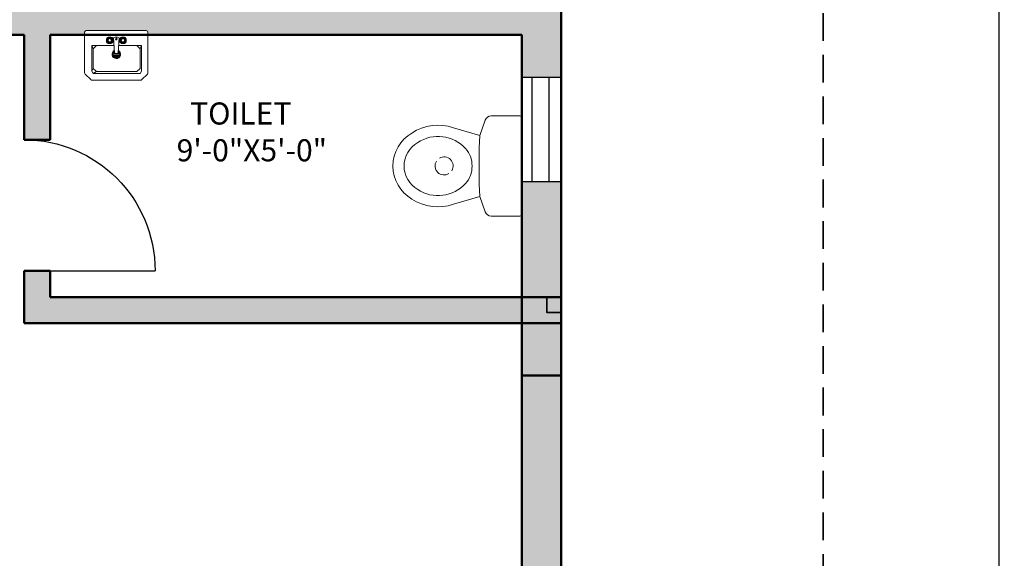
# Model space of a CAD drawing. Units: inches. Extents: x -7 to 1228, y -146 to 1091.
# Tile 86 of 88: x 1003 to 1228, y 691 to 814. Entities that reach past the tile are written whole.
import ezdxf

# ---------------------------------------------------------------- set-up
doc = ezdxf.new("R2010")
doc.units = ezdxf.units.IN
doc.linetypes.add('DASHED2', pattern=[9.525, 6.35, -3.175])
for name, color, linetype, lineweight in [('A-ANNO-DIMS', 2, 'Continuous', 18), ('A-AREA-IDEN', 7, 'Continuous', 18), ('A-COLS', 6, 'Continuous', 35), ('A-DOOR', 4, 'Continuous', 25), ('A-FLOR-FIXT', 8, 'Continuous', 18), ('A-FURN', 8, 'Continuous', 18), ('A-GLAZ', 175, 'Continuous', 25), ('A-WALL', 7, 'Continuous', 50), ('A-WALL-PATT', 251, 'Continuous', 13), ('C-PROP', 1, 'DASHED2', 35)]:
    doc.layers.add(name, color=color, linetype=linetype, lineweight=lineweight)
doc.styles.get("Standard").update_dxf_attribs({"font": 'arial.ttf'})
doc.dimstyles.new('ISO-25', dxfattribs={"dimtxt": 7, "dimasz": 4, "dimexe": 1.25, "dimexo": 0.625, "dimtad": 1, "dimdec": 1, "dimlunit": 3, "dimtxsty": 'Standard', "dimcen": 2.5, "dimadec": 0, "dimazin": 0, "dimtfac": 1, "dimtdec": 1, "dimtmove": 1, "dimatfit": 3, "dimfxl": 1, "dimarcsym": 0})

# ---------------------------------------------------------------- blocks, each defined once
blk = doc.blocks.new('A$C7B5C7CD4')
at = {"ltscale": 20}
for p, q in [((0.243, 0.625), (0.011, 0.625)), ((0.243, 0.625), (0.475, 0.625)), ((0, 0.614), (0, 0.4765)), ((0.486, 0.614), (0.486, 0.4765)), ((0.0212, 0.4467), (0.0946, 0.4214)), ((0.4648, 0.4467), (0.3914, 0.4214)), ((0.0946, 0.4214), (0.0576, 0.293)), ((0.0946, 0.4214), (0.1544, 0.4173)), ((0.3316, 0.4173), (0.1544, 0.4173)), ((0.3914, 0.4214), (0.3316, 0.4173)), ((0.3914, 0.4214), (0.4284, 0.293))]:
    blk.add_line(p, q, dxfattribs=at)
for centre, radius, start, end in [((0.011, 0.614), 0.011, 90, 180), ((0.475, 0.614), 0.011, 0, 90), ((0.0315, 0.4765), 0.0315, 180, 251), ((0.4545, 0.4765), 0.0315, 289, 0), ((0.24, 0.2602), 0.123, 88.6158, 131.7414), ((0.246, 0.2602), 0.123, 48.2586, 91.3842), ((0.2796, 0.219), 0.18, 132.4207, 213.289), ((0.2064, 0.219), 0.18, 326.711, 47.5793), ((0.2796, 0.219), 0.234, 161.5846, 212.8753), ((0.2064, 0.219), 0.234, 327.1247, 18.4154), ((0.243, 0.185), 0.131, 209.6292, 270), ((0.243, 0.185), 0.131, 270, 330.3708), ((0.243, 0.185), 0.185, 210.1745, 270), ((0.243, 0.185), 0.185, 270, 329.8255)]:
    blk.add_arc(centre, radius, start, end, dxfattribs=at)
for start, end in [(58.1785, 211.8215), (238.1785, 31.8215)]:
    blk.add_arc((0.2426, 0.2481), 0.0439, start, end)
blk = doc.blocks.new('*D12')
at = {"layer": 'A-ANNO-DIMS', "color": 0, "lineweight": -2, "transparency": 16777216}
for p, q in [((1187.62, 1061), (1228.45, 1061)), ((1227.2, 1057), (1227.2, 4)), ((1187.62, 0), (1228.45, 0))]:
    blk.add_line(p, q, dxfattribs=at)
at = {"layer": 'A-ANNO-DIMS', "color": 0, "transparency": 16777216}
for points in [[(1226.53, 1057), (1227.86, 1057), (1227.2, 1061)], [(1226.53, 4), (1227.86, 4), (1227.2, 0)]]:
    blk.add_solid(points, dxfattribs=at)
at = {"layer": 'Defpoints', "color": 0, "transparency": 16777216}
for p in [(1187, 1061), (1187, 0), (1227.2, 0)]:
    blk.add_point(p, dxfattribs=at)
at = {"layer": 'A-ANNO-DIMS', "color": 0, "transparency": 16777216, "insert": (1223, 530.5), "char_height": 7, "attachment_point": 5, "rotation": 90}
blk.add_mtext('88\'-5"', dxfattribs=at)
blk = doc.blocks.new('A$C4CB854FF')
for p, q in [((0.4725, 0.38), (0.0125, 0.38)), ((0, 0.3675), (0, 0.0552)), ((0.1677, 0.2932), (0.1677, 0.318)), ((0.1745, 0.2919), (0.1745, 0.3194)), ((0.1773, 0.3221), (0.2048, 0.3221)), ((0.1787, 0.329), (0.2034, 0.329)), ((0.2075, 0.3194), (0.2075, 0.2919)), ((0.2144, 0.318), (0.2144, 0.2932)), ((0.2279, 0.2104), (0.2213, 0.3235)), ((0.2337, 0.329), (0.2502, 0.329)), ((0.2625, 0.3235), (0.256, 0.2104)), ((0.2694, 0.318), (0.2694, 0.2932)), ((0.2763, 0.3194), (0.2763, 0.2919)), ((0.3065, 0.3221), (0.279, 0.3221)), ((0.3052, 0.329), (0.2804, 0.329)), ((0.3093, 0.2919), (0.3093, 0.3194)), ((0.3162, 0.2932), (0.3162, 0.318)), ((0.485, 0.0552), (0.485, 0.3675)), ((0.05, 0.265), (0.2247, 0.265)), ((0.06, 0.24), (0.05, 0.265)), ((0.05, 0.07), (0.05, 0.265)), ((0.085, 0.265), (0.06, 0.24)), ((0.06, 0.24), (0.06, 0.09)), ((0.2048, 0.2891), (0.1773, 0.2891)), ((0.2034, 0.2822), (0.1787, 0.2822)), ((0.2591, 0.265), (0.43, 0.265)), ((0.279, 0.2891), (0.3065, 0.2891)), ((0.2804, 0.2822), (0.3052, 0.2822)), ((0.395, 0.265), (0.42, 0.24)), ((0.42, 0.24), (0.43, 0.265)), ((0.42, 0.24), (0.42, 0.09)), ((0.43, 0.07), (0.43, 0.265)), ((0.2152, 0.1984), (0.2694, 0.1984)), ((0.2297, 0.2066), (0.2165, 0.2066)), ((0.2681, 0.1901), (0.2165, 0.1901)), ((0.2272, 0.2149), (0.2208, 0.2149)), ((0.2638, 0.1819), (0.2208, 0.1819)), ((0.2533, 0.1736), (0.2313, 0.1736)), ((0.2505, 0.2052), (0.2334, 0.2052)), ((0.2681, 0.2066), (0.2541, 0.2066)), ((0.2638, 0.2149), (0.2566, 0.2149)), ((0.06, 0.09), (0.085, 0.065)), ((0.42, 0.09), (0.395, 0.065)), ((0.42, 0.09), (0.43, 0.07)), ((0.0037, 0.0463), (0.0463, 0.0037)), ((0.05, 0.07), (0.06, 0.05)), ((0.42, 0.05), (0.06, 0.05)), ((0.085, 0.065), (0.395, 0.065)), ((0.395, 0.065), (0.42, 0.05)), ((0.43, 0.07), (0.42, 0.05)), ((0.4387, 0.0037), (0.4813, 0.0463)), ((0.0552, 0), (0.4298, 0))]:
    blk.add_line(p, q)
for centre, radius in [((0.191, 0.3056), 0.0165), ((0.191, 0.3056), 0.0127), ((0.2419, 0.3152), 0.00688), ((0.2419, 0.3152), 0.00344), ((0.2928, 0.3056), 0.0165), ((0.2928, 0.3056), 0.0127)]:
    blk.add_circle(centre, radius)
for centre, radius, start, end in [((0.0125, 0.3675), 0.0125, 90, 180), ((0.4725, 0.3675), 0.0125, 0, 90), ((0.1787, 0.318), 0.011, 90, 180), ((0.1773, 0.3194), 0.00275, 90, 180), ((0.2034, 0.318), 0.011, 0, 90), ((0.2048, 0.3194), 0.00275, 360, 90), ((0.2329, 0.314), 0.015, 87.19754, 140.72744), ((0.2509, 0.314), 0.015, 39.27256, 92.80246), ((0.2804, 0.318), 0.011, 90, 180), ((0.279, 0.3194), 0.00275, 90, 180), ((0.3052, 0.318), 0.011, 0, 90), ((0.3065, 0.3194), 0.00275, 360, 90), ((0.1787, 0.2932), 0.011, 180, 270), ((0.1773, 0.2919), 0.00275, 180, 270), ((0.2034, 0.2932), 0.011, 270, 0), ((0.2048, 0.2919), 0.00275, 270, 0), ((0.2423, 0.1984), 0.033, 118.68833, 62.86857), ((0.2804, 0.2932), 0.011, 180, 270), ((0.279, 0.2919), 0.00275, 180, 270), ((0.3052, 0.2932), 0.011, 270, 360), ((0.3065, 0.2919), 0.00275, 270, 0), ((0.2423, 0.1984), 0.0271, 124.77581, 57.22467), ((0.2334, 0.2107), 0.0055, 183.3274, 270), ((0.2505, 0.2107), 0.0055, 270, 356.6726), ((0.0125, 0.0552), 0.0125, 180, 225), ((0.0552, 0.0125), 0.0125, 225, 270), ((0.4298, 0.0125), 0.0125, 270, 315), ((0.4725, 0.0552), 0.0125, 315, 0)]:
    blk.add_arc(centre, radius, start, end)
blk = doc.blocks.new('WIN-24')
for p, q in [((0, 0), (0, 24)), ((0, 24), (9, 24)), ((2.34, 0), (2.34, 24)), ((2.34, 24), (6.14, 24)), ((6.14, 24), (6.14, 0)), ((9, 24), (9, 0)), ((9, 0), (0, 0))]:
    blk.add_line(p, q)
blk = doc.blocks.new('DOOR-750')
blk.add_line((30, 30), (30, 0))
blk.add_arc((30, 30), 30, 180, 270)

msp = doc.modelspace()

# ---------------------------------------------------------------- hatches: boundary and pattern name
at = {"layer": 'A-COLS'}
h = msp.add_hatch(color=256, dxfattribs=at)
h.dxf.hatch_style = 1
h.paths.add_polyline_path([(1127, 747.45), (1123.71, 747.45), (1123.71, 751), (1118, 751), (1118, 733), (1127, 733)])
h = msp.add_hatch(color=256, dxfattribs=at)
h.dxf.hatch_style = 1
h.paths.add_polyline_path([(1127, 747.45), (1127, 751), (1123.71, 751), (1123.71, 747.45)])
at = {"layer": 'A-WALL-PATT'}
h = msp.add_hatch(color=256, dxfattribs=at)
h.dxf.hatch_style = 1
h.paths.add_polyline_path([(69, 568), (60, 568), (60, 493), (63.29, 493), (69, 493)])
h.paths.add_polyline_path([(69, 662.41), (60, 662.41), (60, 586), (69, 586)], flags=17)
h.paths.add_polyline_path([(69, 723), (184, 723), (184, 734), (179, 734), (179, 728), (69, 728), (69, 741.62), (60, 741.62), (60, 698.41), (69, 698.41)], flags=17)
h.paths.add_polyline_path([(69, 782), (231, 782), (231, 728), (231, 723), (231, 586), (236, 586), (236, 787), (69, 787), (69, 800.13), (60, 800.13), (60, 765.62), (69, 765.62)])
h.paths.add_polyline_path([(184, 842), (189, 842), (189, 848), (173, 848), (173, 842), (179, 842), (179, 787), (184, 787)])
h.paths.add_polyline_path([(118.22, 69), (69, 69), (69, 60), (118.22, 60)])
h.paths.add_polyline_path([(227, 69), (154.22, 69), (154.22, 60), (227, 60)])
h.paths.add_polyline_path([(236, 60), (232.71, 60), (227, 60), (227, 36), (236, 36)])
h.paths.add_polyline_path([(389, 60), (380, 60), (380, 36), (389, 36)])
h.paths.add_polyline_path([(384, 181), (380, 181), (380, 115), (380, 78), (384, 78)])
h.paths.add_polyline_path([(380, 115), (334.55, 115), (334.55, 109), (380, 109)])
h.paths.add_polyline_path([(274.55, 115), (236, 115), (236, 201), (232.71, 201), (231, 201), (231, 78), (236, 78), (236, 109), (274.55, 109)])
h.paths.add_polyline_path([(69, 123), (60, 123), (60, 78), (69, 78)])
h.paths.add_polyline_path([(69, 201), (60, 201), (60, 159), (69, 159)])
h.paths.add_polyline_path([(143, 219), (69, 219), (69, 213), (143, 213)], flags=17)
h.paths.add_polyline_path([(189, 219), (184, 219), (184, 274), (231, 274), (231, 219), (236, 219), (236, 279), (184, 279), (184, 297), (179, 297), (179, 279), (69, 279), (69, 290.91), (60, 290.91), (60, 262.18), (69, 262.18), (69, 274), (179, 274), (179, 219), (173, 219), (173, 213), (189, 213)])
h.paths.add_polyline_path([(69, 238.18), (60, 238.18), (60, 219), (69, 219)], flags=17)
h.paths.add_polyline_path([(69, 333), (60, 333), (60, 314.91), (69, 314.91), (69, 316.96)])
h.paths.add_polyline_path([(190, 338), (184, 338), (69, 338), (69, 333), (179, 333), (179, 327), (184, 327), (184, 333.02), (190, 333.05)])
h.paths.add_polyline_path([(69, 386.81), (60, 386.81), (60, 351), (69, 351)])
h.paths.add_polyline_path([(69, 475), (60, 475), (60, 422.81), (69, 422.81)])
h.paths.add_polyline_path([(236, 475), (231, 475), (231, 351.24), (236, 351.24)])
h.paths.add_polyline_path([(384, 475), (380, 475), (380, 362), (384, 362)])
h.paths.add_polyline_path([(547, 307), (439, 307), (439, 356), (445, 356), (445, 362), (433, 362), (433, 307), (380, 307), (380, 244), (380, 241), (384, 241), (384, 301), (433, 301), (433, 277), (439, 277), (439, 301), (547, 301)])
h.paths.add_polyline_path([(547, 241), (439, 241), (439, 247), (433, 247), (433, 235), (547, 235)])
h.paths.add_polyline_path([(450, 69), (440.29, 69), (424.89, 69), (389, 69), (389, 60), (450, 60)])
h.paths.add_polyline_path([(547, 69), (486, 69), (486, 60), (547, 60)])
h.paths.add_polyline_path([(556, 148.27), (547, 148.27), (547, 78), (556, 78)])
h.paths.add_polyline_path([(556, 223), (547, 223), (547, 195), (547, 184.27), (556, 184.27)])
h.paths.add_polyline_path([(556, 311.19), (547, 311.19), (547, 273.08), (556, 273.08)])
h.paths.add_polyline_path([(556, 344), (552.71, 344), (547, 344), (547, 335.19), (556, 335.19)])
h.paths.add_polyline_path([(556, 249.08), (547, 249.08), (547, 241), (556, 241)])
h.paths.add_polyline_path([(547, 362), (475, 362), (475, 356), (547, 356)], flags=0)
h.paths.add_polyline_path([(556, 399.62), (547, 399.62), (547, 362), (556, 362)])
h.paths.add_polyline_path([(556, 475), (547, 475), (547, 435.62), (556, 435.62)])
h.paths.add_polyline_path([(547, 493), (389, 493), (389, 487), (547, 487)])
h.paths.add_polyline_path([(380, 493), (278, 493), (278, 487), (380, 487)])
h.paths.add_polyline_path([(227, 493), (69, 493), (69, 487), (227, 487)])
h.paths.add_polyline_path([(643, 122.44), (634, 122.44), (634, 78), (643, 78)])
h.paths.add_polyline_path([(702.5, 69), (692.79, 69), (677.39, 69), (643, 69), (643, 60), (702.5, 60)])
h.paths.add_polyline_path([(798, 69), (738.5, 69), (738.5, 60), (798, 60)])
h.paths.add_polyline_path([(807, 60), (803.71, 60), (798, 60), (798, 36), (807, 36)])
h.paths.add_polyline_path([(807, 109), (846.75, 109), (846.75, 115), (807, 115), (807, 159), (802, 159), (802, 78), (807, 78)])
h.paths.add_polyline_path([(807, 201), (802, 201), (802, 195), (807, 195)])
h.paths.add_polyline_path([(643, 201), (634, 201), (634, 158.44), (643, 158.44)])
h.paths.add_polyline_path([(756, 225), (751, 225), (751, 219), (643, 219), (643, 213), (756, 213)])
h.paths.add_polyline_path([(643, 240.85), (634, 240.85), (634, 219), (643, 219)])
h.paths.add_polyline_path([(643, 274), (643, 288.63), (634, 288.63), (634, 264.85), (643, 264.85)])
h.paths.add_polyline_path([(802, 279), (756, 279), (756, 297), (751, 297), (751, 279), (643, 279), (643, 274), (751, 274), (751, 255), (756, 255), (756, 274), (802, 274)])
h.paths.add_polyline_path([(807, 333), (803.71, 333), (802, 333), (802, 279), (802, 274), (802, 219), (807, 219)])
h.paths.add_polyline_path([(956, 182), (951, 182), (951, 115), (906.75, 115), (906.75, 109), (951, 109), (951, 78), (956, 78)])
h.paths.add_polyline_path([(960, 60), (951, 60), (951, 36), (960, 36)])
h.paths.add_polyline_path([(1021, 69), (1005.78, 69), (960, 69), (960, 60), (1021, 60)])
h.paths.add_polyline_path([(956, 224), (951, 224), (951, 218), (956, 218)])
h.paths.add_polyline_path([(956, 302), (1004, 302), (1004, 278), (1010, 278), (1010, 302), (1118, 302), (1118, 290.81), (1127, 290.81), (1127, 326.97), (1118, 326.97), (1118, 320.97), (1118, 307), (1010, 307), (1010, 356), (1016, 356), (1016, 362), (1004, 362), (1004, 307), (951, 307), (951, 244), (951, 242), (954.29, 242), (956, 242)])
h.paths.add_polyline_path([(643, 333), (634, 333), (634, 312.63), (643, 312.63), (643, 316.96)])
h.paths.add_polyline_path([(756, 338), (643, 338), (643, 333), (751, 333), (751, 327), (756, 327)])
h.paths.add_polyline_path([(643, 388), (634, 388), (634, 351), (643, 351)])
h.paths.add_polyline_path([(807, 357), (802, 357), (802, 351), (807, 351)])
h.paths.add_polyline_path([(807, 475), (802, 475), (802, 393), (807, 393)])
h.paths.add_polyline_path([(643, 475), (634, 475), (634, 424), (643, 424)])
h.paths.add_polyline_path([(798, 493), (643, 493), (643, 487), (798, 487)])
h.paths.add_polyline_path([(634, 493), (556, 493), (556, 487), (634, 487)])
h.paths.add_polyline_path([(813, 493), (807, 493), (807, 487), (813, 487)])
h.paths.add_polyline_path([(951, 493), (849, 493), (849, 487), (951, 487)])
h.paths.add_polyline_path([(956, 484), (951, 484), (951, 374), (956, 374)])
h.paths.add_polyline_path([(1109, 493), (969, 493), (969, 487), (1109, 487)])
h.paths.add_polyline_path([(1127, 484), (1118, 484), (1118, 450.64), (1127, 450.64)])
h.paths.add_polyline_path([(1127, 414.64), (1118, 414.64), (1118, 365), (1127, 365)])
h.paths.add_polyline_path([(1109, 362), (1046, 362), (1046, 356), (1109, 356)], flags=17)
h.paths.add_polyline_path([(1127, 356), (1123.45, 356), (1118, 356), (1118, 350.97), (1127, 350.97)], flags=0)
h.paths.add_polyline_path([(1127, 266.81), (1118, 266.81), (1118, 262.36), (1118, 242), (1127, 242)], flags=17)
h.paths.add_polyline_path([(1118, 242), (1010, 242), (1010, 248), (1004, 248), (1004, 237), (1118, 237)])
h.paths.add_polyline_path([(1127, 224), (1118, 224), (1118, 170), (1127, 170)])
h.paths.add_polyline_path([(1127, 134), (1118, 134), (1118, 78), (1127, 78)])
h.paths.add_polyline_path([(1118, 69), (1057, 69), (1057, 60), (1118, 60)])
h.paths.add_polyline_path([(227, 571.55), (227, 574), (69, 574), (69, 568), (227, 568)])
h.paths.add_polyline_path([(380, 571.55), (380, 574), (278, 574), (278, 568), (380, 568)])
h.paths.add_polyline_path([(242, 574), (236, 574), (236, 568), (242, 568)])
h.paths.add_polyline_path([(547, 571.55), (547, 574), (389, 574), (389, 568), (547, 568)])
h.paths.add_polyline_path([(384, 733), (380, 733), (380, 586), (384, 586)])
h.paths.add_polyline_path([(556, 646), (634, 646), (634, 655), (547, 655), (547, 586), (556, 586)])
h.paths.add_polyline_path([(634, 574), (556, 574), (556, 568), (634, 568)])
h.paths.add_polyline_path([(643, 655), (634, 655), (634, 586), (643, 586)])
h.paths.add_polyline_path([(798, 574), (643, 574), (643, 568), (798, 568)])
h.paths.add_polyline_path([(643, 663.85), (634, 663.85), (634, 655), (643, 655)])
h.paths.add_polyline_path([(556, 676.97), (547, 676.97), (547, 655), (556, 655)])
h.paths.add_polyline_path([(556, 733), (547, 733), (547, 712.97), (556, 712.97)])
h.paths.add_polyline_path([(643, 710), (634, 710), (634, 699.85), (643, 699.85)])
h.paths.add_polyline_path([(807, 668), (802, 668), (802, 586), (807, 586)])
h.paths.add_polyline_path([(951, 574), (849, 574), (849, 568), (951, 568)])
h.paths.add_polyline_path([(956, 691), (951, 691), (951, 577), (956, 577)])
h.paths.add_polyline_path([(1109, 574), (969, 574), (969, 568), (1109, 568)])
h.paths.add_polyline_path([(1127, 643.4), (1118, 643.4), (1118, 577), (1127, 577)])
h.paths.add_polyline_path([(1127, 568), (1123.45, 568), (1118, 568), (1118, 493), (1127, 493)])
h.paths.add_polyline_path([(1127, 733), (1118, 733), (1118, 679.4), (1127, 679.4)])
h.paths.add_polyline_path([(1127, 777.35), (1118, 777.35), (1118, 770.04), (1118, 751), (1127, 751)], flags=17)
h.paths.add_polyline_path([(1118, 751), (1010, 751), (1010, 757), (1004, 757), (1004, 745), (1118, 745)])
h.paths.add_polyline_path([(956, 811), (1004, 811), (1004, 787), (1010, 787), (1010, 811), (1017.87, 811), (1017.87, 811.63, -0.414214), (1018.25, 812), (1031.98, 812, -0.414214), (1032.35, 811.63), (1032.35, 811), (1118, 811), (1118, 801.35), (1127, 801.35), (1127, 834.69), (1118, 834.69), (1118, 830.24), (1118, 817), (1010, 817), (1010, 866), (1016, 866), (1016, 872), (1004, 872), (1004, 817), (956, 817), (956, 866), (951, 866), (951, 751), (954.29, 751), (956, 751)])
h.paths.add_polyline_path([(1118, 872), (1046, 872), (1046, 866), (1118, 866)], flags=17)
h.paths.add_polyline_path([(1127, 924.71), (1118, 924.71), (1118, 884), (1127, 884)])
h.paths.add_polyline_path([(1127, 866), (1123.71, 866), (1118, 866), (1118, 858.69), (1127, 858.69)], flags=17)
h.paths.add_polyline_path([(956, 983), (951, 983), (951, 952), (807, 952), (807, 983), (802, 983), (802, 902), (807, 902), (807, 946), (951, 946), (951, 884), (956, 884)])
h.paths.add_polyline_path([(807, 842), (802, 842), (802, 787), (756, 787), (756, 806), (751, 806), (751, 787), (643, 787), (643, 782), (751, 782), (751, 764), (756, 764), (756, 782), (802, 782), (802, 728), (807, 728)])
h.paths.add_polyline_path([(756, 848), (643, 848), (643, 842), (751, 842), (751, 836), (756, 836)])
h.paths.add_polyline_path([(756, 734), (751, 734), (751, 728), (643, 728), (643, 723), (756, 723)])
h.paths.add_polyline_path([(643, 749.79), (634, 749.79), (634, 728), (637.29, 728), (643, 728)])
h.paths.add_polyline_path([(643, 805.41), (634, 805.41), (634, 773.79), (643, 773.79)])
h.paths.add_polyline_path([(643, 896.66), (634, 896.66), (634, 860), (637.29, 860), (643, 860)])
h.paths.add_polyline_path([(643, 842), (634, 842), (634, 829.41), (643, 829.41)])
h.paths.add_polyline_path([(643, 983), (634, 983), (634, 932.66), (643, 932.66)])
h.paths.add_polyline_path([(1127, 983), (1118, 983), (1118, 960.71), (1127, 960.71)])
h.paths.add_polyline_path([(1118, 1001), (1077.53, 1001), (1077.53, 992), (1118, 992)])
h.paths.add_polyline_path([(1041.53, 1001), (960, 1001), (960, 992), (1041.53, 992)])
h.paths.add_polyline_path([(960, 1025), (951, 1025), (951, 1001), (954.29, 1001), (960, 1001)])
h.paths.add_polyline_path([(807, 1025), (798, 1025), (798, 1001), (807, 1001)])
h.paths.add_polyline_path([(798, 1001), (738.5, 1001), (738.5, 992), (798, 992)])
h.paths.add_polyline_path([(702.5, 1001), (643, 1001), (643, 992), (702.5, 992)])
h.paths.add_polyline_path([(547, 1001), (499.11, 1001), (499.11, 992), (547, 992)])
h.paths.add_polyline_path([(463.11, 1001), (389, 1001), (389, 992), (463.11, 992)])
h.paths.add_polyline_path([(389, 1025), (380, 1025), (380, 1022), (380, 1001), (383.29, 1001), (389, 1001)])
h.paths.add_polyline_path([(236, 1025), (227, 1025), (227, 1001), (236, 1001)])
h.paths.add_polyline_path([(236, 983), (231, 983), (231, 860), (236, 860)])
h.paths.add_polyline_path([(274.55, 952), (236, 952), (236, 946), (274.55, 946)])
h.paths.add_polyline_path([(380, 952), (334.55, 952), (334.55, 946), (380, 946)])
h.paths.add_polyline_path([(384, 983), (380, 983), (380, 884), (383.29, 884), (384, 884)])
h.paths.add_polyline_path([(227, 1001), (155.01, 1001), (155.01, 992), (162.87, 992), (227, 992)])
h.paths.add_polyline_path([(119.01, 1001), (69, 1001), (69, 992), (119.01, 992)])
h.paths.add_polyline_path([(69, 983), (60, 983), (60, 922.99), (69, 922.99)])
h.paths.add_polyline_path([(69, 886.99), (60, 886.99), (60, 860), (63.29, 860), (69, 860)])
h.paths.add_polyline_path([(143, 848), (69, 848), (69, 842), (143, 842)])

# ---------------------------------------------------------------- linework, layer by layer
at = {"layer": 'A-COLS'}
msp.add_lwpolyline([(1127, 751), (1123.71, 751), (1123.71, 747.45), (1127, 747.45)], close=True, dxfattribs=at)
at = {"layer": 'A-WALL'}
for p, q in [((1127, 60), (1127, 1001)), ((1004, 811), (956, 811)), ((1004, 787), (1004, 811)), ((1118, 811), (1010, 811)), ((1010, 787), (1010, 811)), ((1118, 307), (1118, 811)), ((1010, 787), (1004, 787)), ((1004, 745), (1004, 757)), ((1010, 757), (1004, 757)), ((1010, 751), (1010, 757)), ((1127, 751), (1010, 751)), ((1127, 751), (1118, 751)), ((1118, 751), (1118, 733)), ((1127, 733), (1127, 751)), ((1127, 745), (1004, 745)), ((1118, 733), (1127, 733))]:
    msp.add_line(p, q, dxfattribs=at)
at = {"layer": 'C-PROP'}
msp.add_line((1187, 0), (1187, 1061), dxfattribs=at)

# ---------------------------------------------------------------- block references
at = {"layer": 'A-DOOR', "extrusion": (0, 0, -1), "zscale": -1, "rotation": 269.9999999999974}
msp.add_blockref('DOOR-750', (-1034, 787), dxfattribs=at)
at = {"layer": 'A-FLOR-FIXT', "xscale": 47.26153857112405, "yscale": 47.26153857112405, "zscale": 47.26153857112405, "rotation": 270}
msp.add_blockref('A$C7B5C7CD4', (1088.46, 792.48), dxfattribs=at)
at = {"layer": 'A-FURN', "xscale": -29.84864686937646, "yscale": 29.84864686937646, "zscale": 29.84864686937646}
msp.add_blockref('A$C4CB854FF', (1032.35, 800.66), dxfattribs=at)
at = {"layer": 'A-GLAZ'}
msp.add_blockref('WIN-24', (1118, 777.35), dxfattribs=at)

# ---------------------------------------------------------------- texts
at = {"layer": 'A-AREA-IDEN', "insert": (1038.93, 795.55), "char_height": 5.0568, "attachment_point": 1}
msp.add_mtext_dynamic_manual_height_columns('  TOILET\\P9\'-0"X5\'-0"', width=137.2821, gutter_width=25.28, heights=[0], dxfattribs=at)

# ---------------------------------------------------------------- dimensions: what is measured, and where the dimension line sits
at = {"layer": 'A-ANNO-DIMS'}
dim = msp.add_linear_dim(base=(1227.2, 0), p1=(1187, 1061), p2=(1187, 0), angle=90, dimstyle='ISO-25', override={"dimclrd": 0, "dimclre": 0, "dimclrt": 0}, dxfattribs=at)
dim.commit()
dim.dimension.update_dxf_attribs({"geometry": '*D12', "text_midpoint": (1223, 530.5)})

doc.saveas('drawing.dxf')
